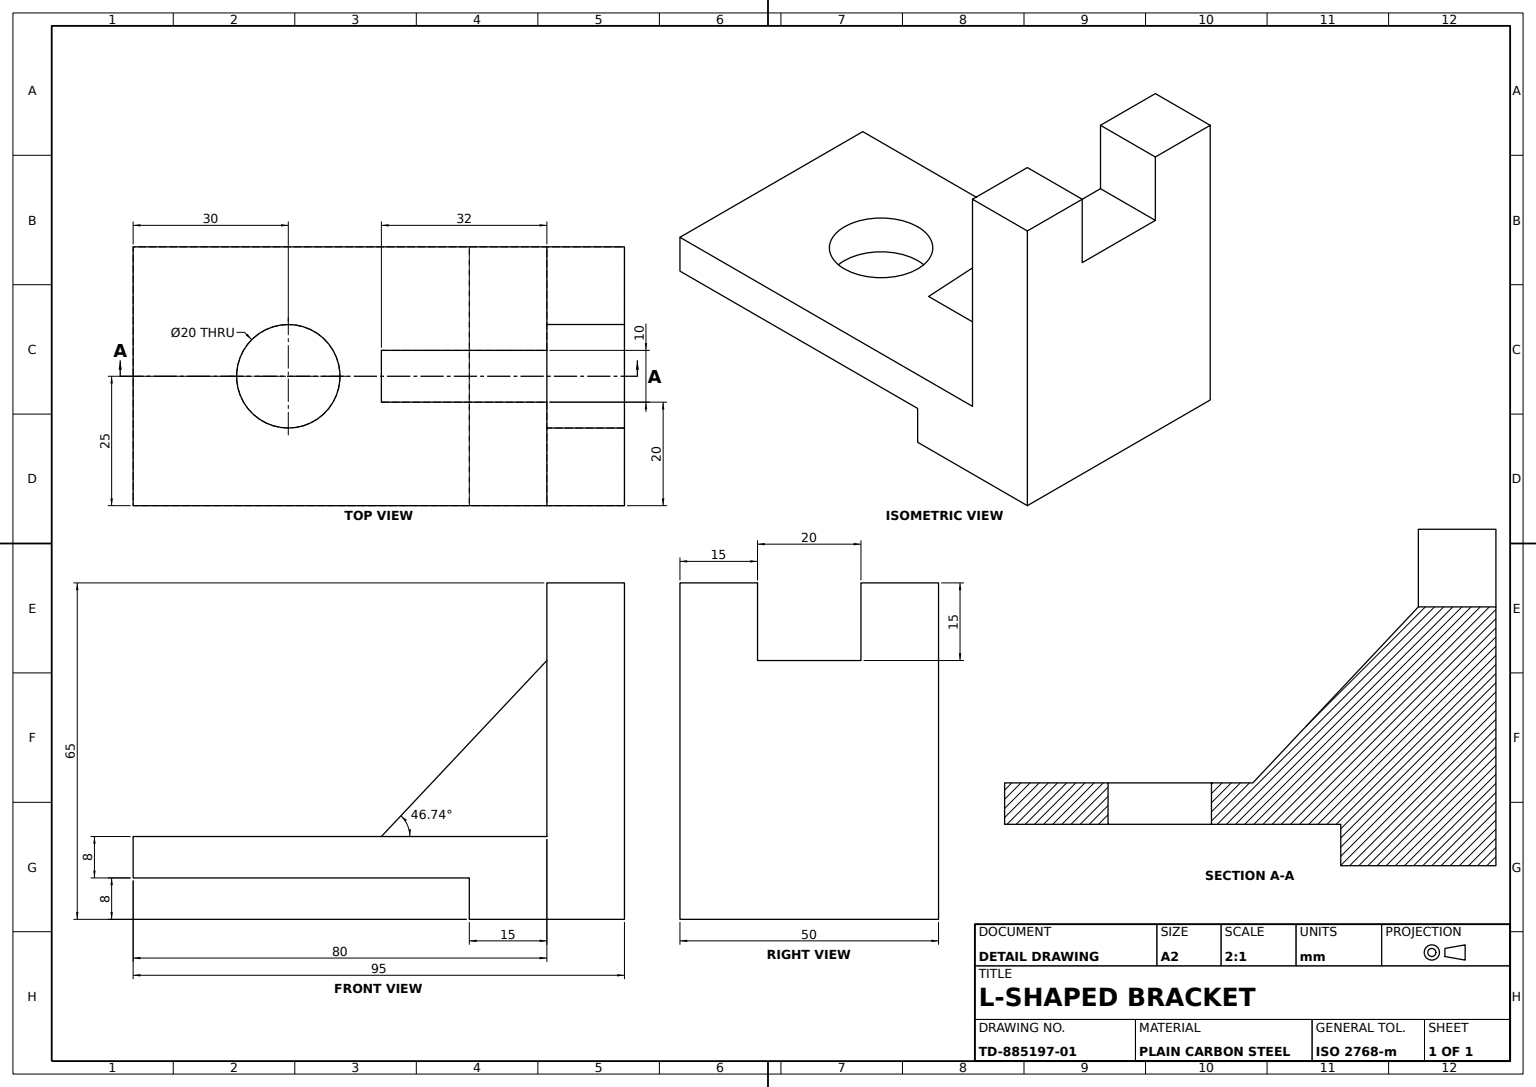
from build123d import *

# Parameters (mm, degrees)
ANGLE_BRACKET_BODY_DEPTH      = 25
ANGLE_BRACKET_BODY_DEPTH_BACK = 25
TOP_SLOT_SKETCH_W             = 20
TOP_SLOT_SKETCH_H             = 15
TOP_SLOT_DEPTH                = 15
MOUNTING_HOLE_SKETCH_R        = 10
BASE_MOUNTING_HOLE_DEPTH      = 8
GUSSET_RIB_DEPTH              = 5


with BuildPart() as part:
    # Bracket L-Profile Sketch → Angle Bracket Body (new, two sides: drawn at the far end of the back side and taken through both)
    with BuildSketch(Plane.XY.offset(-ANGLE_BRACKET_BODY_DEPTH_BACK)):
        Polygon((0, 0), (-30, 0), (-30, 8), (-95, 8), (-95, 16), (-15, 16), (-15, 65), (0, 65), align=None)
    extrude(amount=ANGLE_BRACKET_BODY_DEPTH + ANGLE_BRACKET_BODY_DEPTH_BACK)

    # Top Slot Sketch → Top Slot (cut)
    with BuildSketch(Plane.ZY.offset(15)):
        with Locations((0, 57.5)):
            Rectangle(TOP_SLOT_SKETCH_W, TOP_SLOT_SKETCH_H)
    extrude(amount=-TOP_SLOT_DEPTH, mode=Mode.SUBTRACT)

    # Mounting Hole Sketch → Base Mounting Hole (cut)
    with BuildSketch(Plane(origin=(0, 16, 0), x_dir=(1, 0, 0), z_dir=(0, 1, 0))):
        with Locations(Location((-65, 0, 0), (0, 0, 270))):
            Circle(MOUNTING_HOLE_SKETCH_R)
    extrude(amount=-BASE_MOUNTING_HOLE_DEPTH, mode=Mode.SUBTRACT)

    # Gusset Sketch → Gusset Rib (add, symmetric)
    with BuildSketch(Plane.XY):
        Polygon((-15, 50), (-47, 16), (-15, 16), align=None)
    extrude(amount=GUSSET_RIB_DEPTH, both=True)


solid = part.part
